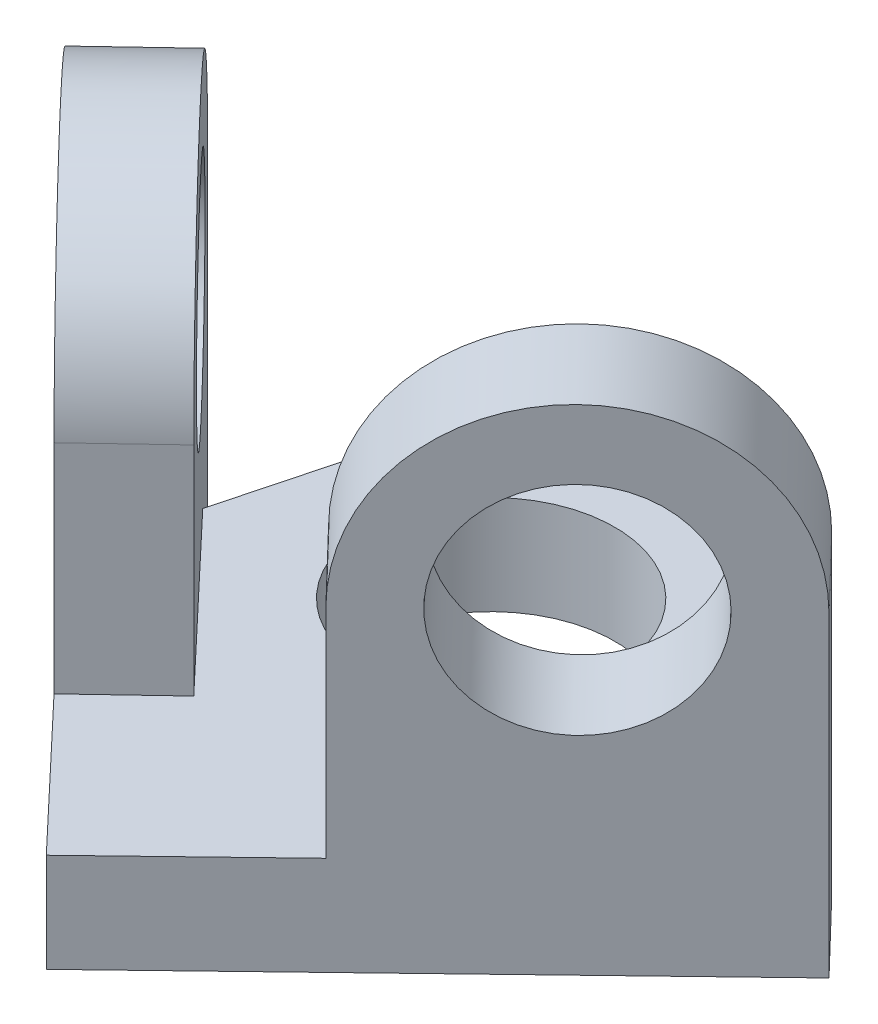
ISO-10303-21;
HEADER;
FILE_DESCRIPTION(('STEP AP214'),'2;1');
FILE_NAME('part.step','',(''),(''),'','','');
FILE_SCHEMA(('AUTOMOTIVE_DESIGN { 1 0 10303 214 1 1 1 1 }'));
ENDSEC;
DATA;
#1=APPLICATION_CONTEXT('core data for automotive mechanical design processes');
#2=APPLICATION_PROTOCOL_DEFINITION('international standard','automotive_design',2000,#1);
#3=PRODUCT_CONTEXT('',#1,'mechanical');
#4=PRODUCT('Part','Part','',(#3));
#5=PRODUCT_RELATED_PRODUCT_CATEGORY('part','',(#4));
#6=PRODUCT_DEFINITION_FORMATION('','',#4);
#7=PRODUCT_DEFINITION_CONTEXT('part definition',#1,'design');
#8=PRODUCT_DEFINITION('design','',#6,#7);
#9=PRODUCT_DEFINITION_SHAPE('','',#8);
#10=(LENGTH_UNIT() NAMED_UNIT(*) SI_UNIT(.MILLI.,.METRE.));
#11=(NAMED_UNIT(*) PLANE_ANGLE_UNIT() SI_UNIT($,.RADIAN.));
#12=(NAMED_UNIT(*) SI_UNIT($,.STERADIAN.) SOLID_ANGLE_UNIT());
#13=UNCERTAINTY_MEASURE_WITH_UNIT(LENGTH_MEASURE(1.E-05),#10,'distance_accuracy_value','');
#14=(GEOMETRIC_REPRESENTATION_CONTEXT(3) GLOBAL_UNCERTAINTY_ASSIGNED_CONTEXT((#13)) GLOBAL_UNIT_ASSIGNED_CONTEXT((#10,
#11,#12)) REPRESENTATION_CONTEXT('',''));
#15=CARTESIAN_POINT('',(0.,0.,0.));
#16=DIRECTION('',(0.,0.,1.));
#17=DIRECTION('',(1.,0.,0.));
#18=AXIS2_PLACEMENT_3D('',#15,#16,#17);
#19=CARTESIAN_POINT('',(-19.336184956302,10.,21.1719042894052));
#20=DIRECTION('',(0.966809247815102,0.,0.25549927267841));
#21=DIRECTION('',(0.25549927267841,0.,-0.966809247815102));
#22=AXIS2_PLACEMENT_3D('',#19,#20,#21);
#23=PLANE('',#22);
#24=DIRECTION('',(0.,-1.,0.));
#25=VECTOR('',#24,1.);
#26=CARTESIAN_POINT('',(-22.460660911913,10.,32.9949213054372));
#27=LINE('',#26,#25);
#28=CARTESIAN_POINT('',(-22.460660911913,10.,32.9949213054372));
#29=VERTEX_POINT('',#28);
#30=CARTESIAN_POINT('',(-22.460660911913,0.,32.9949213054372));
#31=VERTEX_POINT('',#30);
#32=EDGE_CURVE('E50',#29,#31,#27,.T.);
#33=ORIENTED_EDGE('',*,*,#32,.F.);
#34=DIRECTION('',(-0.25549927267841,0.,0.966809247815102));
#35=VECTOR('',#34,1.);
#36=CARTESIAN_POINT('',(-19.336184956302,10.,21.1719042894052));
#37=LINE('',#36,#35);
#38=CARTESIAN_POINT('',(-19.336184956302,10.,21.1719042894052));
#39=VERTEX_POINT('',#38);
#40=EDGE_CURVE('E216',#39,#29,#37,.T.);
#41=ORIENTED_EDGE('',*,*,#40,.F.);
#42=DIRECTION('',(0.,-1.,0.));
#43=VECTOR('',#42,1.);
#44=CARTESIAN_POINT('',(-19.336184956302,10.,21.1719042894052));
#45=LINE('',#44,#43);
#46=CARTESIAN_POINT('',(-19.336184956302,0.,21.1719042894052));
#47=VERTEX_POINT('',#46);
#48=EDGE_CURVE('E238',#39,#47,#45,.T.);
#49=ORIENTED_EDGE('',*,*,#48,.T.);
#50=DIRECTION('',(-0.25549927267841,0.,0.966809247815102));
#51=VECTOR('',#50,1.);
#52=CARTESIAN_POINT('',(-19.336184956302,0.,21.1719042894052));
#53=LINE('',#52,#51);
#54=EDGE_CURVE('E229',#47,#31,#53,.T.);
#55=ORIENTED_EDGE('',*,*,#54,.T.);
#56=EDGE_LOOP('',(#33,#41,#49,#55));
#57=FACE_BOUND('',#56,.T.);
#58=ADVANCED_FACE('F39',(#57),#23,.F.);
#59=CARTESIAN_POINT('',(18.7702426819682,10.,19.3769647136903));
#60=DIRECTION('',(-0.93851213409841,0.,0.345246251464152));
#61=DIRECTION('',(0.345246251464152,0.,0.93851213409841));
#62=AXIS2_PLACEMENT_3D('',#59,#60,#61);
#63=PLANE('',#62);
#64=DIRECTION('',(0.,1.,0.));
#65=VECTOR('',#64,1.);
#66=CARTESIAN_POINT('',(24.1929581888678,10.,34.1179916804011));
#67=LINE('',#66,#65);
#68=CARTESIAN_POINT('',(24.1929581888678,0.,34.1179916804011));
#69=VERTEX_POINT('',#68);
#70=CARTESIAN_POINT('',(24.1929581888678,10.,34.1179916804011));
#71=VERTEX_POINT('',#70);
#72=EDGE_CURVE('E244',#69,#71,#67,.T.);
#73=ORIENTED_EDGE('',*,*,#72,.F.);
#74=DIRECTION('',(-0.345246251464152,0.,-0.93851213409841));
#75=VECTOR('',#74,1.);
#76=CARTESIAN_POINT('',(18.7702426819682,0.,19.3769647136903));
#77=LINE('',#76,#75);
#78=CARTESIAN_POINT('',(18.7702426819682,0.,19.3769647136903));
#79=VERTEX_POINT('',#78);
#80=EDGE_CURVE('E220',#69,#79,#77,.T.);
#81=ORIENTED_EDGE('',*,*,#80,.T.);
#82=DIRECTION('',(0.,-1.,0.));
#83=VECTOR('',#82,1.);
#84=CARTESIAN_POINT('',(18.7702426819682,10.,19.3769647136903));
#85=LINE('',#84,#83);
#86=CARTESIAN_POINT('',(18.7702426819682,10.,19.3769647136903));
#87=VERTEX_POINT('',#86);
#88=EDGE_CURVE('E223',#87,#79,#85,.T.);
#89=ORIENTED_EDGE('',*,*,#88,.F.);
#90=DIRECTION('',(-0.345246251464152,0.,-0.93851213409841));
#91=VECTOR('',#90,1.);
#92=CARTESIAN_POINT('',(18.7702426819682,10.,19.3769647136903));
#93=LINE('',#92,#91);
#94=EDGE_CURVE('E224',#71,#87,#93,.T.);
#95=ORIENTED_EDGE('',*,*,#94,.F.);
#96=EDGE_LOOP('',(#73,#81,#89,#95));
#97=FACE_BOUND('',#96,.T.);
#98=ADVANCED_FACE('F283',(#97),#63,.F.);
#99=CARTESIAN_POINT('',(0.,10.,26.2818897429734));
#100=DIRECTION('',(0.,1.,0.));
#101=DIRECTION('',(0.,0.,1.));
#102=AXIS2_PLACEMENT_3D('',#99,#100,#101);
#103=PLANE('',#102);
#104=DIRECTION('',(0.726370503526785,0.,-0.687303347588417));
#105=VECTOR('',#104,1.);
#106=CARTESIAN_POINT('',(8.71959258808662,10.,35.4971145501567));
#107=LINE('',#106,#105);
#108=CARTESIAN_POINT('',(-13.7460669517683,10.,56.7544796724376));
#109=VERTEX_POINT('',#108);
#110=CARTESIAN_POINT('',(-6.48236191650049,10.,49.8814461965535));
#111=VERTEX_POINT('',#110);
#112=EDGE_CURVE('E11',#109,#111,#107,.T.);
#113=ORIENTED_EDGE('',*,*,#112,.F.);
#114=DIRECTION('',(0.687303347588417,0.,0.726370503526785));
#115=VECTOR('',#114,1.);
#116=CARTESIAN_POINT('',(-25.4662575997213,10.,44.3680991721036));
#117=LINE('',#116,#115);
#118=CARTESIAN_POINT('',(0.,10.,71.2818897429733));
#119=VERTEX_POINT('',#118);
#120=EDGE_CURVE('E218',#109,#119,#117,.T.);
#121=ORIENTED_EDGE('',*,*,#120,.T.);
#122=DIRECTION('',(0.720502211038311,0.,-0.693452639975438));
#123=VECTOR('',#122,1.);
#124=CARTESIAN_POINT('',(0.,10.,71.2818897429733));
#125=LINE('',#124,#123);
#126=CARTESIAN_POINT('',(14.4100442207662,10.,57.4128369434646));
#127=VERTEX_POINT('',#126);
#128=EDGE_CURVE('E222',#119,#127,#125,.T.);
#129=ORIENTED_EDGE('',*,*,#128,.T.);
#130=DIRECTION('',(0.693452639975439,0.,0.720502211038311));
#131=VECTOR('',#130,1.);
#132=CARTESIAN_POINT('',(-8.07349299510335,10.,34.0522823184653));
#133=LINE('',#132,#131);
#134=CARTESIAN_POINT('',(7.47551782101185,10.,50.2078148330815));
#135=VERTEX_POINT('',#134);
#136=EDGE_CURVE('E248',#135,#127,#133,.T.);
#137=ORIENTED_EDGE('',*,*,#136,.F.);
#138=DIRECTION('',(0.720502211038311,0.,-0.693452639975439));
#139=VECTOR('',#138,1.);
#140=CARTESIAN_POINT('',(15.5490108161152,10.,42.4374222575895));
#141=LINE('',#140,#139);
#142=EDGE_CURVE('E200',#135,#71,#141,.T.);
#143=ORIENTED_EDGE('',*,*,#142,.T.);
#144=ORIENTED_EDGE('',*,*,#94,.T.);
#145=CARTESIAN_POINT('',(0.,10.,26.2818897429734));
#146=DIRECTION('',(0.,1.,0.));
#147=DIRECTION('',(0.,0.,1.));
#148=AXIS2_PLACEMENT_3D('',#145,#146,#147);
#149=CIRCLE('',#148,20.);
#150=EDGE_CURVE('E213',#87,#39,#149,.T.);
#151=ORIENTED_EDGE('',*,*,#150,.T.);
#152=ORIENTED_EDGE('',*,*,#40,.T.);
#153=DIRECTION('',(0.687303347588417,0.,0.726370503526785));
#154=VECTOR('',#153,1.);
#155=CARTESIAN_POINT('',(-15.2019545045871,10.,40.6662213893702));
#156=LINE('',#155,#154);
#157=EDGE_CURVE('E53',#29,#111,#156,.T.);
#158=ORIENTED_EDGE('',*,*,#157,.T.);
#159=EDGE_LOOP('',(#113,#121,#129,#137,#143,#144,#151,#152,#158));
#160=FACE_BOUND('',#159,.T.);
#161=CARTESIAN_POINT('',(0.,10.,26.2818897429734));
#162=DIRECTION('',(0.,1.,0.));
#163=DIRECTION('',(0.,0.,1.));
#164=AXIS2_PLACEMENT_3D('',#161,#162,#163);
#165=CIRCLE('',#164,12.5);
#166=CARTESIAN_POINT('',(0.,10.,38.7818897429734));
#167=VERTEX_POINT('',#166);
#168=EDGE_CURVE('E210',#167,#167,#165,.T.);
#169=ORIENTED_EDGE('',*,*,#168,.F.);
#170=EDGE_LOOP('',(#169));
#171=FACE_BOUND('',#170,.T.);
#172=ADVANCED_FACE('F287',(#160,#171),#103,.T.);
#173=CARTESIAN_POINT('',(0.,0.,26.2818897429734));
#174=DIRECTION('',(0.,1.,0.));
#175=DIRECTION('',(0.,0.,1.));
#176=AXIS2_PLACEMENT_3D('',#173,#174,#175);
#177=PLANE('',#176);
#178=DIRECTION('',(0.687303347588417,0.,0.726370503526785));
#179=VECTOR('',#178,1.);
#180=CARTESIAN_POINT('',(-25.4662575997213,0.,44.3680991721036));
#181=LINE('',#180,#179);
#182=CARTESIAN_POINT('',(-38.4889874649513,0.,30.6051415454734));
#183=VERTEX_POINT('',#182);
#184=CARTESIAN_POINT('',(0.,0.,71.2818897429733));
#185=VERTEX_POINT('',#184);
#186=EDGE_CURVE('E230',#183,#185,#181,.T.);
#187=ORIENTED_EDGE('',*,*,#186,.F.);
#188=DIRECTION('',(-0.726370503526785,0.,0.687303347588417));
#189=VECTOR('',#188,1.);
#190=CARTESIAN_POINT('',(-31.2252824296835,0.,23.7321080695892));
#191=LINE('',#190,#189);
#192=CARTESIAN_POINT('',(-31.2252824296835,0.,23.7321080695892));
#193=VERTEX_POINT('',#192);
#194=EDGE_CURVE('E167',#193,#183,#191,.T.);
#195=ORIENTED_EDGE('',*,*,#194,.F.);
#196=DIRECTION('',(0.687303347588417,0.,0.726370503526785));
#197=VECTOR('',#196,1.);
#198=CARTESIAN_POINT('',(-6.48236191650048,0.,49.8814461965535));
#199=LINE('',#198,#197);
#200=EDGE_CURVE('E137',#193,#31,#199,.T.);
#201=ORIENTED_EDGE('',*,*,#200,.T.);
#202=ORIENTED_EDGE('',*,*,#54,.F.);
#203=CARTESIAN_POINT('',(0.,0.,26.2818897429734));
#204=DIRECTION('',(0.,1.,0.));
#205=DIRECTION('',(0.,0.,1.));
#206=AXIS2_PLACEMENT_3D('',#203,#204,#205);
#207=CIRCLE('',#206,20.);
#208=EDGE_CURVE('E209',#79,#47,#207,.T.);
#209=ORIENTED_EDGE('',*,*,#208,.F.);
#210=ORIENTED_EDGE('',*,*,#80,.F.);
#211=DIRECTION('',(0.720502211038311,0.,-0.693452639975438));
#212=VECTOR('',#211,1.);
#213=CARTESIAN_POINT('',(7.47551782101185,0.,50.2078148330815));
#214=LINE('',#213,#212);
#215=CARTESIAN_POINT('',(33.413597418391,0.,25.2435197939657));
#216=VERTEX_POINT('',#215);
#217=EDGE_CURVE('E182',#69,#216,#214,.T.);
#218=ORIENTED_EDGE('',*,*,#217,.T.);
#219=DIRECTION('',(0.693452639975439,0.,0.720502211038311));
#220=VECTOR('',#219,1.);
#221=CARTESIAN_POINT('',(33.413597418391,0.,25.2435197939657));
#222=LINE('',#221,#220);
#223=CARTESIAN_POINT('',(40.3481238181454,0.,32.4485419043488));
#224=VERTEX_POINT('',#223);
#225=EDGE_CURVE('E188',#216,#224,#222,.T.);
#226=ORIENTED_EDGE('',*,*,#225,.T.);
#227=DIRECTION('',(0.720502211038311,0.,-0.693452639975438));
#228=VECTOR('',#227,1.);
#229=CARTESIAN_POINT('',(0.,0.,71.2818897429733));
#230=LINE('',#229,#228);
#231=EDGE_CURVE('E235',#185,#224,#230,.T.);
#232=ORIENTED_EDGE('',*,*,#231,.F.);
#233=EDGE_LOOP('',(#187,#195,#201,#202,#209,#210,#218,#226,#232));
#234=FACE_BOUND('',#233,.T.);
#235=CARTESIAN_POINT('',(0.,0.,26.2818897429734));
#236=DIRECTION('',(0.,1.,0.));
#237=DIRECTION('',(0.,0.,1.));
#238=AXIS2_PLACEMENT_3D('',#235,#236,#237);
#239=CIRCLE('',#238,12.5);
#240=CARTESIAN_POINT('',(0.,0.,38.7818897429734));
#241=VERTEX_POINT('',#240);
#242=EDGE_CURVE('E206',#241,#241,#239,.T.);
#243=ORIENTED_EDGE('',*,*,#242,.T.);
#244=EDGE_LOOP('',(#243));
#245=FACE_BOUND('',#244,.T.);
#246=ADVANCED_FACE('F252',(#234,#245),#177,.F.);
#247=CARTESIAN_POINT('',(0.,10.,26.2818897429734));
#248=DIRECTION('',(0.,-1.,0.));
#249=DIRECTION('',(0.,0.,-1.));
#250=AXIS2_PLACEMENT_3D('',#247,#248,#249);
#251=CYLINDRICAL_SURFACE('',#250,20.);
#252=ORIENTED_EDGE('',*,*,#208,.T.);
#253=ORIENTED_EDGE('',*,*,#48,.F.);
#254=ORIENTED_EDGE('',*,*,#150,.F.);
#255=ORIENTED_EDGE('',*,*,#88,.T.);
#256=EDGE_LOOP('',(#252,#253,#254,#255));
#257=FACE_BOUND('',#256,.T.);
#258=ADVANCED_FACE('F41',(#257),#251,.T.);
#259=CARTESIAN_POINT('',(-25.4662575997213,10.,44.3680991721036));
#260=DIRECTION('',(0.726370503526785,0.,-0.687303347588417));
#261=DIRECTION('',(-0.687303347588417,0.,-0.726370503526785));
#262=AXIS2_PLACEMENT_3D('',#259,#260,#261);
#263=PLANE('',#262);
#264=ORIENTED_EDGE('',*,*,#120,.F.);
#265=DIRECTION('',(0.,1.,0.));
#266=VECTOR('',#265,1.);
#267=CARTESIAN_POINT('',(-13.7460669517683,32.,56.7544796724376));
#268=LINE('',#267,#266);
#269=CARTESIAN_POINT('',(-13.7460669517683,32.,56.7544796724376));
#270=VERTEX_POINT('',#269);
#271=EDGE_CURVE('E157',#109,#270,#268,.T.);
#272=ORIENTED_EDGE('',*,*,#271,.T.);
#273=CARTESIAN_POINT('',(-26.1175272083598,32.,43.6798106089555));
#274=DIRECTION('',(-0.726370503526785,0.,0.687303347588417));
#275=DIRECTION('',(0.687303347588417,0.,0.726370503526785));
#276=AXIS2_PLACEMENT_3D('',#273,#274,#275);
#277=CIRCLE('',#276,18.);
#278=CARTESIAN_POINT('',(-38.4889874649513,32.,30.6051415454734));
#279=VERTEX_POINT('',#278);
#280=EDGE_CURVE('E150',#270,#279,#277,.T.);
#281=ORIENTED_EDGE('',*,*,#280,.T.);
#282=DIRECTION('',(0.,-1.,0.));
#283=VECTOR('',#282,1.);
#284=CARTESIAN_POINT('',(-38.4889874649513,0.,30.6051415454734));
#285=LINE('',#284,#283);
#286=EDGE_CURVE('E162',#279,#183,#285,.T.);
#287=ORIENTED_EDGE('',*,*,#286,.T.);
#288=ORIENTED_EDGE('',*,*,#186,.T.);
#289=DIRECTION('',(0.,-1.,0.));
#290=VECTOR('',#289,1.);
#291=CARTESIAN_POINT('',(0.,10.,71.2818897429733));
#292=LINE('',#291,#290);
#293=EDGE_CURVE('E240',#119,#185,#292,.T.);
#294=ORIENTED_EDGE('',*,*,#293,.F.);
#295=EDGE_LOOP('',(#264,#272,#281,#287,#288,#294));
#296=FACE_BOUND('',#295,.T.);
#297=CARTESIAN_POINT('',(-26.1175272083598,32.,43.6798106089555));
#298=DIRECTION('',(-0.726370503526785,0.,0.687303347588417));
#299=DIRECTION('',(0.687303347588417,0.,0.726370503526785));
#300=AXIS2_PLACEMENT_3D('',#297,#298,#299);
#301=CIRCLE('',#300,11.);
#302=CARTESIAN_POINT('',(-18.5571903848873,32.,51.6698861477501));
#303=VERTEX_POINT('',#302);
#304=EDGE_CURVE('E258',#303,#303,#301,.T.);
#305=ORIENTED_EDGE('',*,*,#304,.F.);
#306=EDGE_LOOP('',(#305));
#307=FACE_BOUND('',#306,.T.);
#308=ADVANCED_FACE('F268',(#296,#307),#263,.F.);
#309=CARTESIAN_POINT('',(0.,10.,71.2818897429733));
#310=DIRECTION('',(-0.693452639975438,0.,-0.720502211038311));
#311=DIRECTION('',(-0.720502211038311,0.,0.693452639975438));
#312=AXIS2_PLACEMENT_3D('',#309,#310,#311);
#313=PLANE('',#312);
#314=ORIENTED_EDGE('',*,*,#231,.T.);
#315=DIRECTION('',(0.,1.,0.));
#316=VECTOR('',#315,1.);
#317=CARTESIAN_POINT('',(40.3481238181454,10.,32.4485419043488));
#318=LINE('',#317,#316);
#319=CARTESIAN_POINT('',(40.3481238181454,32.,32.4485419043488));
#320=VERTEX_POINT('',#319);
#321=EDGE_CURVE('E175',#224,#320,#318,.T.);
#322=ORIENTED_EDGE('',*,*,#321,.T.);
#323=CARTESIAN_POINT('',(27.3790840194558,32.,44.9306894239067));
#324=DIRECTION('',(0.693452639975439,0.,0.720502211038311));
#325=DIRECTION('',(0.720502211038311,0.,-0.693452639975439));
#326=AXIS2_PLACEMENT_3D('',#323,#324,#325);
#327=CIRCLE('',#326,18.);
#328=CARTESIAN_POINT('',(14.4100442207662,32.,57.4128369434646));
#329=VERTEX_POINT('',#328);
#330=EDGE_CURVE('E195',#320,#329,#327,.T.);
#331=ORIENTED_EDGE('',*,*,#330,.T.);
#332=DIRECTION('',(0.,-1.,0.));
#333=VECTOR('',#332,1.);
#334=CARTESIAN_POINT('',(14.4100442207662,10.,57.4128369434646));
#335=LINE('',#334,#333);
#336=EDGE_CURVE('E185',#329,#127,#335,.T.);
#337=ORIENTED_EDGE('',*,*,#336,.T.);
#338=ORIENTED_EDGE('',*,*,#128,.F.);
#339=ORIENTED_EDGE('',*,*,#293,.T.);
#340=EDGE_LOOP('',(#314,#322,#331,#337,#338,#339));
#341=FACE_BOUND('',#340,.T.);
#342=CARTESIAN_POINT('',(27.3790840194558,32.,44.9306894239067));
#343=DIRECTION('',(0.693452639975439,0.,0.720502211038311));
#344=DIRECTION('',(0.720502211038311,0.,-0.693452639975439));
#345=AXIS2_PLACEMENT_3D('',#342,#343,#344);
#346=CIRCLE('',#345,11.);
#347=CARTESIAN_POINT('',(35.3046083408773,32.,37.3027103841769));
#348=VERTEX_POINT('',#347);
#349=EDGE_CURVE('E171',#348,#348,#346,.T.);
#350=ORIENTED_EDGE('',*,*,#349,.F.);
#351=EDGE_LOOP('',(#350));
#352=FACE_BOUND('',#351,.T.);
#353=ADVANCED_FACE('F269',(#341,#352),#313,.F.);
#354=CARTESIAN_POINT('',(0.,10.,26.2818897429734));
#355=DIRECTION('',(0.,-1.,0.));
#356=DIRECTION('',(0.,0.,-1.));
#357=AXIS2_PLACEMENT_3D('',#354,#355,#356);
#358=CYLINDRICAL_SURFACE('',#357,12.5);
#359=ORIENTED_EDGE('',*,*,#168,.T.);
#360=EDGE_LOOP('',(#359));
#361=FACE_BOUND('',#360,.T.);
#362=ORIENTED_EDGE('',*,*,#242,.F.);
#363=EDGE_LOOP('',(#362));
#364=FACE_BOUND('',#363,.T.);
#365=ADVANCED_FACE('F279',(#361,#364),#358,.F.);
#366=CARTESIAN_POINT('',(7.47551782101185,10.,50.2078148330815));
#367=DIRECTION('',(-0.720502211038311,0.,0.693452639975439));
#368=DIRECTION('',(0.693452639975439,0.,0.720502211038311));
#369=AXIS2_PLACEMENT_3D('',#366,#367,#368);
#370=PLANE('',#369);
#371=DIRECTION('',(0.,-1.,0.));
#372=VECTOR('',#371,1.);
#373=CARTESIAN_POINT('',(7.47551782101185,10.,50.2078148330815));
#374=LINE('',#373,#372);
#375=CARTESIAN_POINT('',(7.47551782101186,32.,50.2078148330815));
#376=VERTEX_POINT('',#375);
#377=EDGE_CURVE('E176',#376,#135,#374,.T.);
#378=ORIENTED_EDGE('',*,*,#377,.T.);
#379=ORIENTED_EDGE('',*,*,#136,.T.);
#380=ORIENTED_EDGE('',*,*,#336,.F.);
#381=DIRECTION('',(0.693452639975439,0.,0.720502211038311));
#382=VECTOR('',#381,1.);
#383=CARTESIAN_POINT('',(7.47551782101186,32.,50.2078148330815));
#384=LINE('',#383,#382);
#385=EDGE_CURVE('E197',#376,#329,#384,.T.);
#386=ORIENTED_EDGE('',*,*,#385,.F.);
#387=EDGE_LOOP('',(#378,#379,#380,#386));
#388=FACE_BOUND('',#387,.T.);
#389=ADVANCED_FACE('F300',(#388),#370,.T.);
#390=CARTESIAN_POINT('',(20.4445576197015,32.,37.7256673135236));
#391=DIRECTION('',(0.693452639975439,0.,0.720502211038311));
#392=DIRECTION('',(0.720502211038311,0.,-0.693452639975439));
#393=AXIS2_PLACEMENT_3D('',#390,#391,#392);
#394=CYLINDRICAL_SURFACE('',#393,18.);
#395=ORIENTED_EDGE('',*,*,#330,.F.);
#396=DIRECTION('',(0.693452639975439,0.,0.720502211038311));
#397=VECTOR('',#396,1.);
#398=CARTESIAN_POINT('',(33.413597418391,32.,25.2435197939657));
#399=LINE('',#398,#397);
#400=CARTESIAN_POINT('',(33.413597418391,32.,25.2435197939657));
#401=VERTEX_POINT('',#400);
#402=EDGE_CURVE('E199',#401,#320,#399,.T.);
#403=ORIENTED_EDGE('',*,*,#402,.F.);
#404=CARTESIAN_POINT('',(20.4445576197015,32.,37.7256673135236));
#405=DIRECTION('',(0.693452639975439,0.,0.720502211038311));
#406=DIRECTION('',(0.720502211038311,0.,-0.693452639975439));
#407=AXIS2_PLACEMENT_3D('',#404,#405,#406);
#408=CIRCLE('',#407,18.);
#409=EDGE_CURVE('E186',#401,#376,#408,.T.);
#410=ORIENTED_EDGE('',*,*,#409,.T.);
#411=ORIENTED_EDGE('',*,*,#385,.T.);
#412=EDGE_LOOP('',(#395,#403,#410,#411));
#413=FACE_BOUND('',#412,.T.);
#414=ADVANCED_FACE('F308',(#413),#394,.T.);
#415=CARTESIAN_POINT('',(33.413597418391,10.,25.2435197939657));
#416=DIRECTION('',(0.720502211038311,0.,-0.693452639975439));
#417=DIRECTION('',(-0.693452639975439,0.,-0.720502211038311));
#418=AXIS2_PLACEMENT_3D('',#415,#416,#417);
#419=PLANE('',#418);
#420=ORIENTED_EDGE('',*,*,#321,.F.);
#421=ORIENTED_EDGE('',*,*,#225,.F.);
#422=DIRECTION('',(0.,1.,0.));
#423=VECTOR('',#422,1.);
#424=CARTESIAN_POINT('',(33.413597418391,10.,25.2435197939657));
#425=LINE('',#424,#423);
#426=EDGE_CURVE('E184',#216,#401,#425,.T.);
#427=ORIENTED_EDGE('',*,*,#426,.T.);
#428=ORIENTED_EDGE('',*,*,#402,.T.);
#429=EDGE_LOOP('',(#420,#421,#427,#428));
#430=FACE_BOUND('',#429,.T.);
#431=ADVANCED_FACE('F305',(#430),#419,.T.);
#432=CARTESIAN_POINT('',(20.4445576197015,32.,37.7256673135236));
#433=DIRECTION('',(0.693452639975439,0.,0.720502211038311));
#434=DIRECTION('',(0.720502211038311,0.,-0.693452639975439));
#435=AXIS2_PLACEMENT_3D('',#432,#433,#434);
#436=PLANE('',#435);
#437=ORIENTED_EDGE('',*,*,#142,.F.);
#438=ORIENTED_EDGE('',*,*,#377,.F.);
#439=ORIENTED_EDGE('',*,*,#409,.F.);
#440=ORIENTED_EDGE('',*,*,#426,.F.);
#441=ORIENTED_EDGE('',*,*,#217,.F.);
#442=ORIENTED_EDGE('',*,*,#72,.T.);
#443=EDGE_LOOP('',(#437,#438,#439,#440,#441,#442));
#444=FACE_BOUND('',#443,.T.);
#445=CARTESIAN_POINT('',(20.4445576197015,32.,37.7256673135236));
#446=DIRECTION('',(0.693452639975439,0.,0.720502211038311));
#447=DIRECTION('',(0.720502211038311,0.,-0.693452639975439));
#448=AXIS2_PLACEMENT_3D('',#445,#446,#447);
#449=CIRCLE('',#448,11.);
#450=CARTESIAN_POINT('',(28.3700819411229,32.,30.0976882737938));
#451=VERTEX_POINT('',#450);
#452=EDGE_CURVE('E172',#451,#451,#449,.T.);
#453=ORIENTED_EDGE('',*,*,#452,.T.);
#454=EDGE_LOOP('',(#453));
#455=FACE_BOUND('',#454,.T.);
#456=ADVANCED_FACE('F302',(#444,#455),#436,.F.);
#457=CARTESIAN_POINT('',(20.4445576197015,32.,37.7256673135236));
#458=DIRECTION('',(0.693452639975439,0.,0.720502211038311));
#459=DIRECTION('',(0.720502211038311,0.,-0.693452639975439));
#460=AXIS2_PLACEMENT_3D('',#457,#458,#459);
#461=CYLINDRICAL_SURFACE('',#460,11.);
#462=ORIENTED_EDGE('',*,*,#452,.F.);
#463=EDGE_LOOP('',(#462));
#464=FACE_BOUND('',#463,.T.);
#465=ORIENTED_EDGE('',*,*,#349,.T.);
#466=EDGE_LOOP('',(#465));
#467=FACE_BOUND('',#466,.T.);
#468=ADVANCED_FACE('F316',(#464,#467),#461,.F.);
#469=CARTESIAN_POINT('',(-31.2252824296835,0.,23.7321080695892));
#470=DIRECTION('',(-0.687303347588417,0.,-0.726370503526785));
#471=DIRECTION('',(-0.726370503526785,0.,0.687303347588417));
#472=AXIS2_PLACEMENT_3D('',#469,#470,#471);
#473=PLANE('',#472);
#474=ORIENTED_EDGE('',*,*,#286,.F.);
#475=DIRECTION('',(-0.726370503526785,0.,0.687303347588417));
#476=VECTOR('',#475,1.);
#477=CARTESIAN_POINT('',(-31.2252824296835,32.,23.7321080695892));
#478=LINE('',#477,#476);
#479=CARTESIAN_POINT('',(-31.2252824296835,32.,23.7321080695892));
#480=VERTEX_POINT('',#479);
#481=EDGE_CURVE('E146',#480,#279,#478,.T.);
#482=ORIENTED_EDGE('',*,*,#481,.F.);
#483=DIRECTION('',(0.,-1.,0.));
#484=VECTOR('',#483,1.);
#485=CARTESIAN_POINT('',(-31.2252824296835,0.,23.7321080695892));
#486=LINE('',#485,#484);
#487=EDGE_CURVE('E149',#480,#193,#486,.T.);
#488=ORIENTED_EDGE('',*,*,#487,.T.);
#489=ORIENTED_EDGE('',*,*,#194,.T.);
#490=EDGE_LOOP('',(#474,#482,#488,#489));
#491=FACE_BOUND('',#490,.T.);
#492=ADVANCED_FACE('F317',(#491),#473,.T.);
#493=CARTESIAN_POINT('',(-18.853822173092,32.,36.8067771330713));
#494=DIRECTION('',(-0.726370503526785,0.,0.687303347588417));
#495=DIRECTION('',(0.687303347588417,0.,0.726370503526785));
#496=AXIS2_PLACEMENT_3D('',#493,#494,#495);
#497=CYLINDRICAL_SURFACE('',#496,18.);
#498=ORIENTED_EDGE('',*,*,#280,.F.);
#499=DIRECTION('',(-0.726370503526785,0.,0.687303347588417));
#500=VECTOR('',#499,1.);
#501=CARTESIAN_POINT('',(-6.48236191650049,32.,49.8814461965535));
#502=LINE('',#501,#500);
#503=CARTESIAN_POINT('',(-6.48236191650049,32.,49.8814461965535));
#504=VERTEX_POINT('',#503);
#505=EDGE_CURVE('E135',#504,#270,#502,.T.);
#506=ORIENTED_EDGE('',*,*,#505,.F.);
#507=CARTESIAN_POINT('',(-18.853822173092,32.,36.8067771330713));
#508=DIRECTION('',(-0.726370503526785,0.,0.687303347588417));
#509=DIRECTION('',(0.687303347588417,0.,0.726370503526785));
#510=AXIS2_PLACEMENT_3D('',#507,#508,#509);
#511=CIRCLE('',#510,18.);
#512=EDGE_CURVE('E139',#504,#480,#511,.T.);
#513=ORIENTED_EDGE('',*,*,#512,.T.);
#514=ORIENTED_EDGE('',*,*,#481,.T.);
#515=EDGE_LOOP('',(#498,#506,#513,#514));
#516=FACE_BOUND('',#515,.T.);
#517=ADVANCED_FACE('F145',(#516),#497,.T.);
#518=CARTESIAN_POINT('',(-6.48236191650049,32.,49.8814461965535));
#519=DIRECTION('',(0.687303347588417,0.,0.726370503526785));
#520=DIRECTION('',(0.726370503526785,0.,-0.687303347588417));
#521=AXIS2_PLACEMENT_3D('',#518,#519,#520);
#522=PLANE('',#521);
#523=ORIENTED_EDGE('',*,*,#271,.F.);
#524=ORIENTED_EDGE('',*,*,#112,.T.);
#525=DIRECTION('',(0.,1.,0.));
#526=VECTOR('',#525,1.);
#527=CARTESIAN_POINT('',(-6.48236191650049,32.,49.8814461965535));
#528=LINE('',#527,#526);
#529=EDGE_CURVE('E131',#111,#504,#528,.T.);
#530=ORIENTED_EDGE('',*,*,#529,.T.);
#531=ORIENTED_EDGE('',*,*,#505,.T.);
#532=EDGE_LOOP('',(#523,#524,#530,#531));
#533=FACE_BOUND('',#532,.T.);
#534=ADVANCED_FACE('F133',(#533),#522,.T.);
#535=CARTESIAN_POINT('',(-18.853822173092,32.,36.8067771330713));
#536=DIRECTION('',(-0.726370503526785,0.,0.687303347588417));
#537=DIRECTION('',(0.687303347588417,0.,0.726370503526785));
#538=AXIS2_PLACEMENT_3D('',#535,#536,#537);
#539=PLANE('',#538);
#540=ORIENTED_EDGE('',*,*,#157,.F.);
#541=ORIENTED_EDGE('',*,*,#32,.T.);
#542=ORIENTED_EDGE('',*,*,#200,.F.);
#543=ORIENTED_EDGE('',*,*,#487,.F.);
#544=ORIENTED_EDGE('',*,*,#512,.F.);
#545=ORIENTED_EDGE('',*,*,#529,.F.);
#546=EDGE_LOOP('',(#540,#541,#542,#543,#544,#545));
#547=FACE_BOUND('',#546,.T.);
#548=CARTESIAN_POINT('',(-18.853822173092,32.,36.8067771330713));
#549=DIRECTION('',(-0.726370503526785,0.,0.687303347588417));
#550=DIRECTION('',(0.687303347588417,0.,0.726370503526785));
#551=AXIS2_PLACEMENT_3D('',#548,#549,#550);
#552=CIRCLE('',#551,11.);
#553=CARTESIAN_POINT('',(-11.2934853496194,32.,44.796852671866));
#554=VERTEX_POINT('',#553);
#555=EDGE_CURVE('E161',#554,#554,#552,.T.);
#556=ORIENTED_EDGE('',*,*,#555,.T.);
#557=EDGE_LOOP('',(#556));
#558=FACE_BOUND('',#557,.T.);
#559=ADVANCED_FACE('F151',(#547,#558),#539,.F.);
#560=CARTESIAN_POINT('',(-18.853822173092,32.,36.8067771330713));
#561=DIRECTION('',(-0.726370503526785,0.,0.687303347588417));
#562=DIRECTION('',(0.687303347588417,0.,0.726370503526785));
#563=AXIS2_PLACEMENT_3D('',#560,#561,#562);
#564=CYLINDRICAL_SURFACE('',#563,11.);
#565=ORIENTED_EDGE('',*,*,#555,.F.);
#566=EDGE_LOOP('',(#565));
#567=FACE_BOUND('',#566,.T.);
#568=ORIENTED_EDGE('',*,*,#304,.T.);
#569=EDGE_LOOP('',(#568));
#570=FACE_BOUND('',#569,.T.);
#571=ADVANCED_FACE('F265',(#567,#570),#564,.F.);
#572=CLOSED_SHELL('',(#58,#98,#172,#246,#258,#308,#353,#365,#389,#414,#431,#456,#468,#492,#517,
#534,#559,#571));
#573=MANIFOLD_SOLID_BREP('B2',#572);
#574=ADVANCED_BREP_SHAPE_REPRESENTATION('',(#18,#573),#14);
#575=SHAPE_DEFINITION_REPRESENTATION(#9,#574);
ENDSEC;
END-ISO-10303-21;
